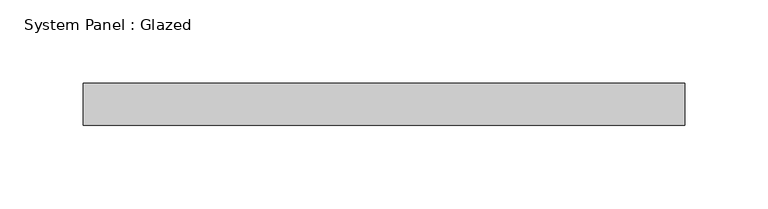
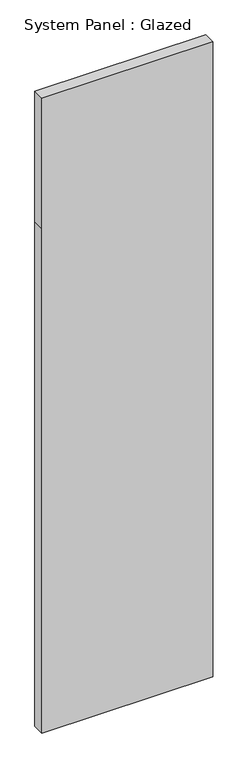
"""IFC4 building model written with IfcOpenShell, lengths in millimetres: plate geometry, System Panel : Glazed."""

from ifc_helpers import new_model, si_unit, frame, origin, place, context, project, spatial, polyline, outline, extrude, source, transform, mapped, element, save


def system_panel_glazed_1627a9b9(model_context):
    return source(origin(), model_context, "Body", "SweptSolid", [
        extrude(outline(polyline([(0.0, -180.975), (0.0, 180.975), (1130.3, 180.975), (1422.4, 180.975), (1422.4, -180.975), (1130.3, -180.975), (0.0, -180.975)])), frame((0.0, 19.05, 0.0), z_axis=(0.0, 1.0, 0.0), x_axis=(0.0, 0.0, 1.0)), (0.0, 0.0, 1.0), 25.4),
    ])


if __name__ == "__main__":
    model = new_model("IFC4")
    model_context = context("Model", 3, world=origin())
    ifc_project = project(units=[si_unit("LENGTHUNIT", "METRE", prefix="MILLI")], contexts=[model_context])
    site = spatial("IfcSite", under=ifc_project)
    building = spatial("IfcBuilding", under=site)
    placement = place(None, origin())
    system_panel_glazed_shape = system_panel_glazed_1627a9b9(model_context)
    element("IfcPlate", 1, ObjectType="System Panel : Glazed", at=placement, inside=building, context=model_context, shape_type="MappedRepresentation", body=[
        mapped(system_panel_glazed_shape, transform((0.0, 0.0, 0.0), x_axis=(1.0, 0.0, 0.0), y_axis=(0.0, 1.0, 0.0), z_axis=(0.0, 0.0, 1.0))),
    ])
    save(model, "model.ifc")

# Revit data of these elements
# Type "System Panel : Glazed"
#   Construction Type Id = "GSP4R"
#   Analytic Construction = "1/8 in Pilkington single glazing"
#   Visual Light Transmittance = 0.9
#   Solar Heat Gain Coefficient = 0.86
#   Heat Transfer Coefficient (U) = 1.18115 BTU/(h·ft²·°F)
#   Define Thermal Properties by = 1
# Element 1 (IfcPlate, "System Panel : Glazed")
#   Materials on its faces: "Glass"
# Materials
#   "Glass": class "Glass", colour RGB 0 128 192, transparency 0.75, Description = "Soda Lime Glass", Cost = 0
